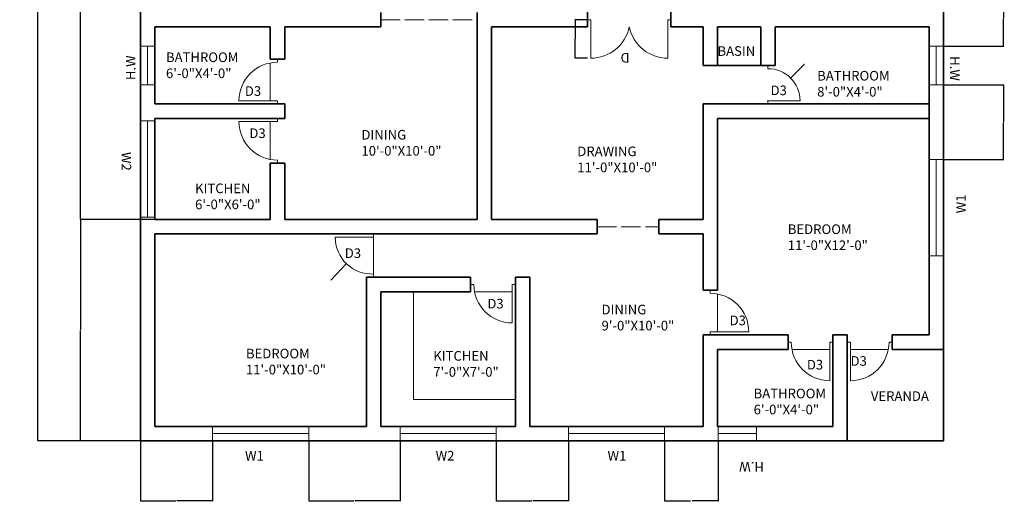
# Model space of a CAD drawing. Units: inches. Extents: x -51 to 563, y -718 to 47.
# Tile 1 of 2: x -51 to 563, y -718 to -418. Entities that reach past the tile are written whole.
import ezdxf

# ---------------------------------------------------------------- set-up
doc = ezdxf.new("R2010")
doc.units = ezdxf.units.IN
doc.header["$MEASUREMENT"] = 0
doc.linetypes.add('ACAD_ISO02W100', pattern=[15, 12, -3])
for name, color, linetype, lineweight in [('A-ANNO-DIMS', 2, 'Continuous', 18), ('A-ANNO-TEXT', 7, 'Continuous', 18), ('A-AREA-IDEN', 7, 'Continuous', 18), ('A-DOOR', 3, 'Continuous', 18), ('A-FLOR-CASE', 9, 'Continuous', 18), ('A-GLAZ', 164, 'Continuous', 18), ('A-WALL', 7, 'Continuous', 35), ('A-WALL-OPEN', 8, 'ACAD_ISO02W100', 13)]:
    doc.layers.add(name, color=color, linetype=linetype, lineweight=lineweight)
doc.styles.get("Standard").update_dxf_attribs({"font": 'arial.ttf'})
doc.dimstyles.get("Standard").update_dxf_attribs({"dimtxt": 0.18, "dimasz": 0.18, "dimexe": 0.18, "dimexo": 0.0625, "dimgap": 0.09, "dimtad": 0, "dimtih": 1, "dimtoh": 1, "dimdec": 0, "dimzin": 0, "dimdsep": 46, "dimlunit": 3, "dimtxsty": 'Standard', "dimcen": 0.09, "dimadec": 0, "dimazin": 0, "dimtfac": 1, "dimtdec": 0, "dimtofl": 0, "dimtmove": 0, "dimatfit": 3, "dimfxl": 1, "dimtolj": 1, "dimtzin": 0, "dimarcsym": 0})

# ---------------------------------------------------------------- blocks, each defined once
blk = doc.blocks.new('*D2')
at = {"layer": 'A-ANNO-DIMS', "color": 0, "lineweight": -2, "transparency": 16777216}
for p, q in [((24.17, 9.71), (-39.93, 9.71)), ((-39.75, 9.53), (-39.75, -332.13)), ((-39.75, -680.11), (-39.75, -338.44)), ((24.17, -680.29), (-39.93, -680.29))]:
    blk.add_line(p, q, dxfattribs=at)
at = {"layer": 'A-ANNO-DIMS', "color": 0, "transparency": 16777216}
for points in [[(-39.78, 9.53), (-39.72, 9.53), (-39.75, 9.71)], [(-39.78, -680.11), (-39.72, -680.11), (-39.75, -680.29)]]:
    blk.add_solid(points, dxfattribs=at)
at = {"layer": 'Defpoints', "color": 0, "transparency": 16777216}
for p in [(24.24, 9.71), (-39.75, -680.29), (24.24, -680.29)]:
    blk.add_point(p, dxfattribs=at)
at = {"layer": 'A-ANNO-DIMS', "color": 0, "transparency": 16777216, "insert": (-39.75, -335.29), "char_height": 6, "attachment_point": 5}
blk.add_mtext('\\A1;57\'-6"', dxfattribs=at)
blk = doc.blocks.new('WIN-60IN')
for p, q in [((0, 9), (60, 9)), ((0, 0), (0, 9)), ((60, 9), (60, 0)), ((0, 4.5), (60, 4.5)), ((60, 0), (0, 0))]:
    blk.add_line(p, q)
blk = doc.blocks.new('WIN-24IN')
for p, q in [((0, 9), (24, 9)), ((0, 0), (0, 9)), ((24, 9), (24, 0)), ((0, 4.5), (24, 4.5)), ((24, 0), (0, 0))]:
    blk.add_line(p, q)
blk = doc.blocks.new('DOOR-24IN-OFFSET-THRESHOLD')
for p, q in [((19.5, 25.57), (19.5, 2)), ((24, 26), (24, 28)), ((24, 2), (0, 2)), ((24, 0), (24, 2))]:
    blk.add_line(p, q)
blk.add_arc((24, 2), 24, 90, 180)
blk = doc.blocks.new('DOOR-48IN-PAIR')
for p, q in [((2, 0), (2, 24)), ((50, 0), (50, 24)), ((0, 0), (2, 0)), ((50, 0), (52, 0))]:
    blk.add_line(p, q)
for centre, start, end in [((2, -0.52), 11.81228, 90), ((50, -0.52), 90, 168.18772)]:
    blk.add_arc(centre, 24.52, start, end)
blk = doc.blocks.new('*D19')
at = {"layer": 'A-ANNO-DIMS', "color": 0, "lineweight": -2, "transparency": 16777216}
for p, q in [((303.24, -417.72), (303.24, -409.81)), ((303.42, -409.99), (327.69, -409.99)), ((355.06, -409.99), (330.79, -409.99)), ((355.24, -417.72), (355.24, -409.81))]:
    blk.add_line(p, q, dxfattribs=at)
at = {"layer": 'A-ANNO-DIMS', "color": 0, "transparency": 16777216}
for points in [[(303.42, -409.96), (303.42, -410.02), (303.24, -409.99)], [(355.06, -409.96), (355.06, -410.02), (355.24, -409.99)]]:
    blk.add_solid(points, dxfattribs=at)
at = {"layer": 'Defpoints', "color": 0, "transparency": 16777216}
for p in [(303.24, -409.99), (303.24, -417.79), (355.24, -417.79)]:
    blk.add_point(p, dxfattribs=at)
at = {"layer": 'A-ANNO-DIMS', "color": 0, "transparency": 16777216, "insert": (329.24, -409.99), "char_height": 0.18, "attachment_point": 5}
blk.add_mtext('\\A1;PAIRED DOOR 4\'-4" TYP.', dxfattribs=at)
blk = doc.blocks.new('*D20')
at = {"layer": 'A-ANNO-DIMS', "color": 0, "lineweight": -2, "transparency": 16777216}
for p, q in [((303.17, -417.79), (295.26, -417.79)), ((295.44, -417.97), (295.44, -429.6)), ((295.44, -441.61), (295.44, -429.97)), ((303.17, -441.79), (295.26, -441.79))]:
    blk.add_line(p, q, dxfattribs=at)
at = {"layer": 'A-ANNO-DIMS', "color": 0, "transparency": 16777216}
for points in [[(295.41, -417.97), (295.47, -417.97), (295.44, -417.79)], [(295.41, -441.61), (295.47, -441.61), (295.44, -441.79)]]:
    blk.add_solid(points, dxfattribs=at)
at = {"layer": 'Defpoints', "color": 0, "transparency": 16777216}
for p in [(303.24, -417.79), (295.44, -441.79), (303.24, -441.79)]:
    blk.add_point(p, dxfattribs=at)
at = {"layer": 'A-ANNO-DIMS', "color": 0, "transparency": 16777216, "insert": (295.44, -429.79), "char_height": 0.18, "attachment_point": 5}
blk.add_mtext('\\A1;2\'-0" TYP.', dxfattribs=at)
blk = doc.blocks.new('*D21')
at = {"layer": 'A-ANNO-DIMS', "color": 0, "lineweight": -2, "transparency": 16777216}
for p, q in [((24.24, -680.35), (24.24, -717.87)), ((69.24, -680.35), (69.24, -717.87)), ((24.42, -717.69), (46.41, -717.69)), ((69.06, -717.69), (47.07, -717.69))]:
    blk.add_line(p, q, dxfattribs=at)
at = {"layer": 'A-ANNO-DIMS', "color": 0, "transparency": 16777216}
for points in [[(24.42, -717.66), (24.42, -717.72), (24.24, -717.69)], [(69.06, -717.66), (69.06, -717.72), (69.24, -717.69)]]:
    blk.add_solid(points, dxfattribs=at)
at = {"layer": 'Defpoints', "color": 0, "transparency": 16777216}
for p in [(24.24, -680.29), (69.24, -680.29), (69.24, -717.69)]:
    blk.add_point(p, dxfattribs=at)
at = {"layer": 'A-ANNO-DIMS', "color": 0, "transparency": 16777216, "insert": (46.74, -717.69), "char_height": 0.18, "attachment_point": 5}
blk.add_mtext('\\A1;3\'-9"', dxfattribs=at)
blk = doc.blocks.new('*D22')
at = {"layer": 'A-ANNO-DIMS', "color": 0, "lineweight": -2, "transparency": 16777216}
for p, q in [((129.24, -680.35), (129.24, -717.87)), ((186.24, -680.35), (186.24, -717.87)), ((129.42, -717.69), (157.4, -717.69)), ((186.06, -717.69), (158.07, -717.69))]:
    blk.add_line(p, q, dxfattribs=at)
at = {"layer": 'A-ANNO-DIMS', "color": 0, "transparency": 16777216}
for points in [[(129.42, -717.66), (129.42, -717.72), (129.24, -717.69)], [(186.06, -717.66), (186.06, -717.72), (186.24, -717.69)]]:
    blk.add_solid(points, dxfattribs=at)
at = {"layer": 'Defpoints', "color": 0, "transparency": 16777216}
for p in [(129.24, -680.29), (186.24, -680.29), (186.24, -717.69)]:
    blk.add_point(p, dxfattribs=at)
at = {"layer": 'A-ANNO-DIMS', "color": 0, "transparency": 16777216, "insert": (157.74, -717.69), "char_height": 0.18, "attachment_point": 5}
blk.add_mtext('\\A1;4\'-9"', dxfattribs=at)
blk = doc.blocks.new('*D23')
at = {"layer": 'A-ANNO-DIMS', "color": 0, "lineweight": -2, "transparency": 16777216}
for p, q in [((246.24, -680.35), (246.24, -717.87)), ((291.24, -680.35), (291.24, -717.87)), ((246.42, -717.69), (268.41, -717.69)), ((291.06, -717.69), (269.07, -717.69))]:
    blk.add_line(p, q, dxfattribs=at)
at = {"layer": 'A-ANNO-DIMS', "color": 0, "transparency": 16777216}
for points in [[(246.42, -717.66), (246.42, -717.72), (246.24, -717.69)], [(291.06, -717.66), (291.06, -717.72), (291.24, -717.69)]]:
    blk.add_solid(points, dxfattribs=at)
at = {"layer": 'Defpoints', "color": 0, "transparency": 16777216}
for p in [(246.24, -680.29), (291.24, -680.29), (291.24, -717.69)]:
    blk.add_point(p, dxfattribs=at)
at = {"layer": 'A-ANNO-DIMS', "color": 0, "transparency": 16777216, "insert": (268.74, -717.69), "char_height": 0.18, "attachment_point": 5}
blk.add_mtext('\\A1;3\'-9"', dxfattribs=at)
blk = doc.blocks.new('*D24')
at = {"layer": 'A-ANNO-DIMS', "color": 0, "lineweight": -2, "transparency": 16777216}
for p, q in [((351.24, -680.35), (351.24, -717.87)), ((384.65, -680.35), (384.65, -717.87)), ((351.42, -717.69), (367.4, -717.69)), ((384.47, -717.69), (368.48, -717.69))]:
    blk.add_line(p, q, dxfattribs=at)
at = {"layer": 'A-ANNO-DIMS', "color": 0, "transparency": 16777216}
for points in [[(351.42, -717.66), (351.42, -717.72), (351.24, -717.69)], [(384.47, -717.66), (384.47, -717.72), (384.65, -717.69)]]:
    blk.add_solid(points, dxfattribs=at)
at = {"layer": 'Defpoints', "color": 0, "transparency": 16777216}
for p in [(351.24, -680.29), (384.65, -680.29), (384.65, -717.69)]:
    blk.add_point(p, dxfattribs=at)
at = {"layer": 'A-ANNO-DIMS', "color": 0, "transparency": 16777216, "insert": (367.94, -717.69), "char_height": 0.18, "attachment_point": 5}
blk.add_mtext('\\A1;2\'-9 1/2"', dxfattribs=at)
blk = doc.blocks.new('*D26')
at = {"layer": 'A-ANNO-DIMS', "color": 0, "lineweight": -2, "transparency": 16777216}
for p, q in [((33.17, -272.29), (-13.34, -272.29)), ((-13.16, -272.47), (-13.16, -407.1)), ((-13.16, -542.11), (-13.16, -407.47)), ((33.17, -542.29), (-13.34, -542.29))]:
    blk.add_line(p, q, dxfattribs=at)
at = {"layer": 'A-ANNO-DIMS', "color": 0, "transparency": 16777216}
for points in [[(-13.19, -272.47), (-13.13, -272.47), (-13.16, -272.29)], [(-13.19, -542.11), (-13.13, -542.11), (-13.16, -542.29)]]:
    blk.add_solid(points, dxfattribs=at)
at = {"layer": 'Defpoints', "color": 0, "transparency": 16777216}
for p in [(33.24, -272.29), (-13.16, -542.29), (33.24, -542.29)]:
    blk.add_point(p, dxfattribs=at)
at = {"layer": 'A-ANNO-DIMS', "color": 0, "transparency": 16777216, "insert": (-13.16, -407.29), "char_height": 0.18, "attachment_point": 5}
blk.add_mtext('\\A1;22\'-6"', dxfattribs=at)
blk = doc.blocks.new('*D27')
at = {"layer": 'A-ANNO-DIMS', "color": 0, "lineweight": -2, "transparency": 16777216}
for p, q in [((33.17, -542.29), (-13.34, -542.29)), ((-13.16, -542.47), (-13.16, -611.1)), ((-13.16, -680.11), (-13.16, -611.47)), ((24.17, -680.29), (-13.34, -680.29))]:
    blk.add_line(p, q, dxfattribs=at)
at = {"layer": 'A-ANNO-DIMS', "color": 0, "transparency": 16777216}
for points in [[(-13.19, -542.47), (-13.13, -542.47), (-13.16, -542.29)], [(-13.19, -680.11), (-13.13, -680.11), (-13.16, -680.29)]]:
    blk.add_solid(points, dxfattribs=at)
at = {"layer": 'Defpoints', "color": 0, "transparency": 16777216}
for p in [(33.24, -542.29), (-13.16, -680.29), (24.24, -680.29)]:
    blk.add_point(p, dxfattribs=at)
at = {"layer": 'A-ANNO-DIMS', "color": 0, "transparency": 16777216, "insert": (-13.16, -611.29), "char_height": 0.18, "attachment_point": 5}
blk.add_mtext('\\A1;11\'-6"', dxfattribs=at)
blk = doc.blocks.new('*D31')
at = {"layer": 'A-ANNO-DIMS', "color": 0, "lineweight": -2, "transparency": 16777216}
for p, q in [((525.3, -399.79), (562.82, -399.79)), ((562.64, -399.97), (562.64, -416.85)), ((562.64, -434.11), (562.64, -417.22)), ((525.3, -434.29), (562.82, -434.29))]:
    blk.add_line(p, q, dxfattribs=at)
at = {"layer": 'A-ANNO-DIMS', "color": 0, "transparency": 16777216}
for points in [[(562.61, -399.97), (562.67, -399.97), (562.64, -399.79)], [(562.61, -434.11), (562.67, -434.11), (562.64, -434.29)]]:
    blk.add_solid(points, dxfattribs=at)
at = {"layer": 'Defpoints', "color": 0, "transparency": 16777216}
for p in [(525.24, -399.79), (525.24, -434.29), (562.64, -434.29)]:
    blk.add_point(p, dxfattribs=at)
at = {"layer": 'A-ANNO-DIMS', "color": 0, "transparency": 16777216, "insert": (562.64, -417.04), "char_height": 0.18, "attachment_point": 5}
blk.add_mtext('\\A1;2\'-10 1/2"', dxfattribs=at)
blk = doc.blocks.new('*D32')
at = {"layer": 'A-ANNO-DIMS', "color": 0, "lineweight": -2, "transparency": 16777216}
for p, q in [((525.3, -458.29), (562.82, -458.29)), ((562.64, -458.47), (562.64, -481.42)), ((562.64, -504.75), (562.64, -481.79)), ((525.3, -504.93), (562.82, -504.93))]:
    blk.add_line(p, q, dxfattribs=at)
at = {"layer": 'A-ANNO-DIMS', "color": 0, "transparency": 16777216}
for points in [[(562.61, -458.47), (562.67, -458.47), (562.64, -458.29)], [(562.61, -504.75), (562.67, -504.75), (562.64, -504.93)]]:
    blk.add_solid(points, dxfattribs=at)
at = {"layer": 'Defpoints', "color": 0, "transparency": 16777216}
for p in [(525.24, -458.29), (525.24, -504.93), (562.64, -504.93)]:
    blk.add_point(p, dxfattribs=at)
at = {"layer": 'A-ANNO-DIMS', "color": 0, "transparency": 16777216, "insert": (562.64, -481.61), "char_height": 0.18, "attachment_point": 5}
blk.add_mtext('\\A1;3\'-10 1/2"', dxfattribs=at)
blk = doc.blocks.new('*D37')
at = {"layer": 'A-ANNO-DIMS', "color": 0, "lineweight": -2, "transparency": 16777216}
for p, q in [((168.67, -553.29), (168.85, -553.29)), ((168.76, -553.38), (168.76, -553.2)), ((143.27, -579.88), (152.7, -570.04)), ((143.09, -579.88), (143.27, -579.88))]:
    blk.add_line(p, q, dxfattribs=at)
at = {"layer": 'A-ANNO-DIMS', "color": 0, "transparency": 16777216}
blk.add_solid([(152.68, -570.02), (152.73, -570.06), (152.83, -569.91)], dxfattribs=at)
at = {"layer": 'Defpoints', "color": 0, "transparency": 16777216}
for p in [(168.76, -553.29), (152.83, -569.91)]:
    blk.add_point(p, dxfattribs=at)
at = {"layer": 'A-ANNO-DIMS', "color": 0, "transparency": 16777216, "insert": (142.61, -579.88), "char_height": 0.18, "attachment_point": 5}
blk.add_mtext('\\A1;R1\'-11"', dxfattribs=at)
blk = doc.blocks.new('*D39')
at = {"layer": 'A-ANNO-DIMS', "color": 0, "lineweight": -2, "transparency": 16777216}
for p, q in [((438.36, -445.66), (430.01, -454.02)), ((438.54, -445.66), (438.36, -445.66)), ((415.65, -468.29), (415.83, -468.29)), ((415.74, -468.38), (415.74, -468.2))]:
    blk.add_line(p, q, dxfattribs=at)
at = {"layer": 'A-ANNO-DIMS', "color": 0, "transparency": 16777216}
blk.add_solid([(429.98, -454), (430.03, -454.04), (429.88, -454.14)], dxfattribs=at)
at = {"layer": 'Defpoints', "color": 0, "transparency": 16777216}
for p in [(429.88, -454.14), (415.74, -468.29)]:
    blk.add_point(p, dxfattribs=at)
at = {"layer": 'A-ANNO-DIMS', "color": 0, "transparency": 16777216, "insert": (438.96, -445.66), "char_height": 0.18, "attachment_point": 5}
blk.add_mtext('\\A1;R1\'-8"', dxfattribs=at)

msp = doc.modelspace()

# ---------------------------------------------------------------- linework, layer by layer
at = {"layer": 'A-DOOR'}
for p, q in [((415.74, -446.29), (415.74, -448.29)), ((415.74, -470.29), (415.74, -468.29)), ((415.74, -468.29), (435.74, -468.29)), ((169.74, -551.29), (169.74, -553.29)), ((169.74, -553.29), (145.74, -553.29)), ((169.74, -553.29), (169.74, -576.29)), ((169.74, -578.29), (169.74, -576.29))]:
    msp.add_line(p, q, dxfattribs=at)
for centre, radius, start, end in [((415.74, -468.29), 20, 0, 90), ((168.76, -553.29), 23.02, 180, 272.43775)]:
    msp.add_arc(centre, radius, start, end, dxfattribs=at)
at = {"layer": 'A-FLOR-CASE'}
for p, q in [((194.67, -587.29), (194.67, -654.51)), ((194.67, -654.51), (258.24, -654.51))]:
    msp.add_line(p, q, dxfattribs=at)
at = {"layer": 'A-WALL'}
for p, q in [((24.24, 9.71), (24.24, -680.29)), ((525.24, -317.29), (525.24, -680.29)), ((174.24, -413.29), (174.24, -422.29)), ((234.24, -422.29), (234.24, -413.29)), ((303.24, -413.29), (303.24, -422.29)), ((355.24, -417.79), (355.24, -413.29)), ((33.24, -422.29), (105.24, -422.29)), ((33.24, -422.29), (33.24, -470.29)), ((105.24, -422.29), (105.24, -442.29)), ((114.24, -422.29), (114.24, -442.29)), ((114.24, -422.29), (174.24, -422.29)), ((234.24, -422.29), (234.24, -470.29)), ((243.24, -422.29), (243.24, -470.29)), ((243.24, -422.29), (303.24, -422.29)), ((355.24, -417.79), (355.24, -422.29)), ((355.24, -422.29), (375.24, -422.29)), ((375.24, -422.29), (375.24, -446.29)), ((384.24, -422.29), (384.24, -446.29)), ((384.24, -422.29), (411.24, -422.29)), ((384.24, -422.29), (384.24, -446.29)), ((411.24, -422.29), (411.24, -446.29)), ((420.24, -422.29), (420.24, -446.29)), ((420.24, -422.29), (516.24, -422.29)), ((516.24, -422.29), (516.24, -614.29)), ((516.24, -422.29), (516.24, -470.29)), ((525.24, -422.29), (525.24, -470.29)), ((109.74, -442.29), (105.24, -442.29)), ((109.74, -442.29), (114.24, -442.29)), ((384.24, -446.29), (375.24, -446.29)), ((384.24, -446.29), (420.24, -446.29)), ((33.24, -470.29), (105.24, -470.29)), ((105.24, -470.29), (114.24, -470.29)), ((114.24, -470.29), (114.24, -479.29)), ((234.24, -470.29), (234.24, -479.29)), ((243.24, -470.29), (243.24, -480.54)), ((375.24, -470.29), (375.24, -479.29)), ((384.24, -470.29), (375.24, -470.29)), ((384.24, -470.29), (516.24, -470.29)), ((33.24, -479.29), (105.24, -479.29)), ((33.24, -479.29), (33.24, -542.29)), ((105.24, -479.29), (114.24, -479.29)), ((234.24, -479.29), (234.24, -542.29)), ((243.24, -479.29), (243.24, -542.29)), ((375.24, -479.29), (375.24, -542.29)), ((384.24, -479.29), (384.24, -542.29)), ((384.24, -479.29), (516.24, -479.29)), ((109.74, -507.29), (105.24, -507.29)), ((105.24, -507.29), (105.24, -542.29)), ((109.74, -507.29), (114.24, -507.29)), ((114.24, -507.29), (114.24, -542.29)), ((33.24, -542.29), (105.24, -542.29)), ((114.24, -542.29), (234.24, -542.29)), ((243.24, -542.29), (309.24, -542.29)), ((309.24, -542.29), (309.24, -551.29)), ((347.6, -542.29), (347.6, -551.29)), ((347.6, -542.29), (375.24, -542.29)), ((384.24, -542.29), (384.24, -551.29)), ((33.24, -551.29), (309.24, -551.29)), ((33.24, -551.29), (33.24, -671.29)), ((347.6, -551.29), (375.24, -551.29)), ((375.24, -551.29), (375.24, -586.29)), ((384.24, -551.29), (384.24, -586.29)), ((165.24, -578.29), (165.24, -671.29)), ((165.24, -578.29), (230.24, -578.29)), ((230.24, -582.79), (230.24, -578.29)), ((230.24, -582.79), (230.24, -587.29)), ((258.24, -578.29), (258.24, -671.29)), ((258.24, -578.29), (267.24, -578.29)), ((267.24, -578.29), (267.24, -671.29)), ((174.24, -587.29), (230.24, -587.29)), ((174.24, -587.29), (174.24, -671.29)), ((379.74, -586.29), (375.24, -586.29)), ((379.74, -586.29), (384.24, -586.29)), ((375.24, -614.29), (428.24, -614.29)), ((375.24, -614.29), (375.24, -671.29)), ((428.24, -618.79), (428.24, -614.29)), ((428.24, -618.79), (428.24, -623.29)), ((456.24, -614.29), (456.24, -671.29)), ((456.24, -614.29), (465.24, -614.29)), ((465.24, -614.29), (465.24, -671.29)), ((493.24, -618.79), (493.24, -614.29)), ((493.24, -614.29), (516.24, -614.29)), ((493.24, -618.79), (493.24, -623.29)), ((384.24, -623.29), (428.24, -623.29)), ((384.24, -623.29), (384.24, -671.29)), ((493.24, -623.29), (525.24, -623.29)), ((33.24, -671.29), (165.24, -671.29)), ((174.24, -671.29), (258.24, -671.29)), ((267.24, -671.29), (375.24, -671.29)), ((384.24, -671.29), (456.24, -671.29)), ((465.24, -671.29), (465.24, -680.29)), ((24.24, -680.29), (465.24, -680.29)), ((465.24, -680.29), (525.24, -680.29))]:
    msp.add_line(p, q, dxfattribs=at)
at = {"layer": 'A-WALL-OPEN'}
for p, q in [((174.24, -417.79), (234.24, -417.79)), ((309.24, -546.79), (347.6, -546.79))]:
    msp.add_line(p, q, dxfattribs=at)

# ---------------------------------------------------------------- block references
at = {"layer": 'A-DOOR'}
for name, p, rotation in [('DOOR-48IN-PAIR', (355.24, -417.79), 180), ('DOOR-24IN-OFFSET-THRESHOLD', (258.24, -606.79), 89.99999999999972), ('DOOR-24IN-OFFSET-THRESHOLD', (456.24, -642.79), 89.99999999999982)]:
    msp.add_blockref(name, p, dxfattribs=dict(at, rotation=rotation))
msp.add_blockref('DOOR-24IN-OFFSET-THRESHOLD', (85.74, -470.29), dxfattribs=at)
at = {"layer": 'A-DOOR', "extrusion": (0, 0, -1), "zscale": -1}
for p, rotation in [((-85.74, -479.29), 180), ((-465.24, -642.79), 89.99999999999969)]:
    msp.add_blockref('DOOR-24IN-OFFSET-THRESHOLD', p, dxfattribs=dict(at, rotation=rotation))
msp.add_blockref('DOOR-24IN-OFFSET-THRESHOLD', (-403.74, -614.29), dxfattribs=at)
at = {"layer": 'A-GLAZ'}
for name, p, rotation in [('WIN-24IN', (24.24, -434.29), 269.9999999999995), ('WIN-24IN', (516.24, -434.29), 269.9999999999995), ('WIN-60IN', (33.24, -540.79), 90.00000000000003), ('WIN-60IN', (525.24, -564.93), 90.00000000000003)]:
    msp.add_blockref(name, p, dxfattribs=dict(at, rotation=rotation))
for name, p in [('WIN-60IN', (69.24, -680.29)), ('WIN-60IN', (186.24, -680.29)), ('WIN-60IN', (291.24, -680.29)), ('WIN-24IN', (384.65, -680.29))]:
    msp.add_blockref(name, p, dxfattribs=at)

# ---------------------------------------------------------------- texts
at = {"layer": 'A-ANNO-TEXT', "char_height": 6, "attachment_point": 1}
for s, insert, rotation in [('H.W', (15.18, -455.42), 90), ('D', (329.4, -444.49), 180), ('H.W', (535.39, -440.48), 270), ('W2', (18.46, -500.22), 270), ('W1', (533.15, -538.45), 90), ('H.W', (413.19, -699.44), 180)]:
    msp.add_mtext(s, dxfattribs=dict(at, insert=insert, rotation=rotation))
for s, insert in [('D3', (89.4, -459.24)), ('D3', (417.35, -458.8)), ('D3', (92.21, -485.52)), ('D3', (151.74, -560.31)), ('D3', (240.66, -591.76)), ('D3', (391.81, -602.2)), ('D3', (439.99, -629.8)), ('D3', (467.24, -627.49)), ('W1', (89.53, -686.54)), ('W2', (208.42, -686.54)), ('W1', (315.66, -686.54))]:
    msp.add_mtext(s, dxfattribs=dict(at, insert=insert))
at = {"layer": 'A-AREA-IDEN', "char_height": 6, "attachment_point": 1}
for s, insert in [('BASIN', (384.24, -434.29)), ('BATHROOM\\P6\'-0"X4\'-0"', (40.19, -438.18)), ('BATHROOM\\P8\'-0"X4\'-0"', (446.43, -449.69)), ('DINING\\P10\'-0"X10\'-0"', (162.13, -486.5)), ('DRAWING\\P11\'-0"X10\'-0"', (296.78, -496.83)), ('KITCHEN\\P6\'-0"X6\'-0"', (58.35, -519.9)), ('BEDROOM\\P11\'-0"X12\'-0"', (428.1, -545.36)), ('DINING\\P9\'-0"X10\'-0"', (311.91, -595.45)), ('BEDROOM\\P11\'-0"X10\'-0"', (90.08, -622.86)), ('KITCHEN\\P7\'-0"X7\'-0"', (206.94, -624.31)), ('BATHROOM\\P6\'-0"X4\'-0"', (406.78, -647.76)), ('VERANDA', (479.91, -649.4))]:
    msp.add_mtext(s, dxfattribs=dict(at, insert=insert))

# ---------------------------------------------------------------- dimensions: what is measured, and where the dimension line sits
at = {"layer": 'A-ANNO-DIMS'}
for base, p1, p2, override, picture, middle in [((-39.75, -680.29), (24.24, 9.71), (24.24, -680.29), {"dimtxt": 6, "dimclrd": 0, "dimclre": 0, "dimclrt": 0}, '*D2', (-39.75, -335.29)), ((-13.16, -542.29), (33.24, -272.29), (33.24, -542.29), {"dimdec": 1, "dimlfac": 1, "dimrnd": 0, "dimzin": 1, "dimdsep": 46, "dimlunit": 4, "dimfrac": 2}, '*D26', (-13.16, -407.29)), ((562.64, -434.29), (525.24, -399.79), (525.24, -434.29), {"dimdec": 1, "dimlfac": 1, "dimrnd": 0, "dimzin": 1, "dimdsep": 46, "dimlunit": 4, "dimfrac": 2}, '*D31', (562.64, -417.04)), ((562.64, -504.93), (525.24, -458.29), (525.24, -504.93), {"dimdec": 1, "dimlfac": 1, "dimrnd": 0, "dimzin": 1, "dimdsep": 46, "dimlunit": 4, "dimfrac": 2}, '*D32', (562.64, -481.61)), ((-13.16, -680.29), (33.24, -542.29), (24.24, -680.29), {"dimdec": 1, "dimlfac": 1, "dimrnd": 0, "dimzin": 1, "dimdsep": 46, "dimlunit": 4, "dimfrac": 2}, '*D27', (-13.16, -611.29))]:
    dim = msp.add_linear_dim(base=base, p1=p1, p2=p2, angle=90, dimstyle='Standard', override=override, dxfattribs=at)
    dim.commit()
    dim.dimension.update_dxf_attribs({"geometry": picture, "text_midpoint": middle})
for base, p1, p2, angle, text, picture, middle in [((303.24, -409.99), (355.24, -417.79), (303.24, -417.79), 180, 'PAIRED DOOR <> TYP.', '*D19', (329.24, -409.99)), ((295.44, -441.79), (303.24, -417.79), (303.24, -441.79), 270, '<> TYP.', '*D20', (295.44, -429.79))]:
    dim = msp.add_linear_dim(base=base, p1=p1, p2=p2, angle=angle, text=text, dimstyle='Standard', override={"dimdec": 1, "dimlfac": 1, "dimrnd": 0, "dimzin": 1, "dimdsep": 46, "dimlunit": 4, "dimfrac": 2}, dxfattribs=at)
    dim.commit()
    dim.dimension.update_dxf_attribs({"geometry": picture, "text_midpoint": middle})
for center, mpoint, picture, middle in [((415.74, -468.29), (429.88, -454.14), '*D39', (438.96, -445.66)), ((168.76, -553.29), (152.83, -569.91), '*D37', (142.61, -579.88))]:
    dim = msp.add_radius_dim(center=center, mpoint=mpoint, dimstyle='Standard', override={"dimdec": 1, "dimlfac": 1, "dimrnd": 0, "dimzin": 1, "dimdsep": 46, "dimlunit": 4, "dimfrac": 2}, dxfattribs=at)
    dim.commit()
    dim.dimension.update_dxf_attribs({"geometry": picture, "text_midpoint": middle, "dimtype": 164})
for base, p1, p2, picture, middle in [((69.24, -717.69), (24.24, -680.29), (69.24, -680.29), '*D21', (46.74, -717.69)), ((186.24, -717.69), (129.24, -680.29), (186.24, -680.29), '*D22', (157.74, -717.69)), ((291.24, -717.69), (246.24, -680.29), (291.24, -680.29), '*D23', (268.74, -717.69)), ((384.65, -717.69), (351.24, -680.29), (384.65, -680.29), '*D24', (367.94, -717.69))]:
    dim = msp.add_linear_dim(base=base, p1=p1, p2=p2, dimstyle='Standard', override={"dimdec": 1, "dimlfac": 1, "dimrnd": 0, "dimzin": 1, "dimdsep": 46, "dimlunit": 4, "dimfrac": 2}, dxfattribs=at)
    dim.commit()
    dim.dimension.update_dxf_attribs({"geometry": picture, "text_midpoint": middle})

doc.saveas('drawing.dxf')
